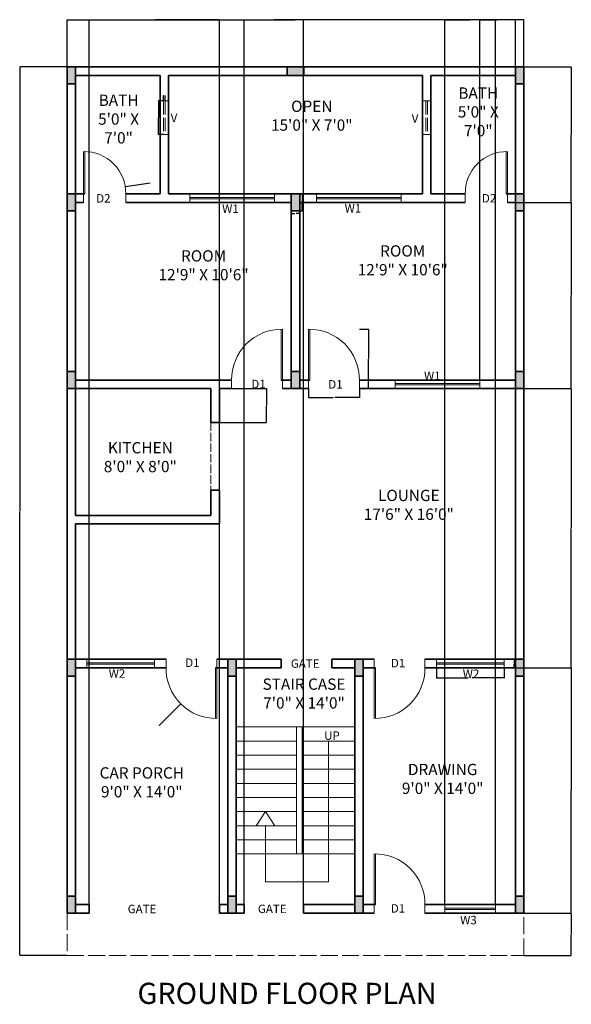
# Model space of a CAD drawing. Units: inches. Extents: x -1239 to -402, y 1021 to 1720.
# Tile 1 of 2: x -1239 to -847, y 1021 to 1720. Entities that reach past the tile are written whole.
import ezdxf

# ---------------------------------------------------------------- set-up
doc = ezdxf.new("R2010")
doc.units = ezdxf.units.IN
doc.linetypes.add('ACAD_ISO02W100', pattern=[15, 12, -3])
for name, color, linetype, lineweight in [('A-ANNO-DIMS', 2, 'Continuous', 18), ('A-ANNO-SYMB', 7, 'Continuous', 18), ('A-ANNO-TEXT', 7, 'Continuous', 18), ('A-ANNO-TITL', 7, 'Continuous', 35), ('A-AREA-IDEN', 7, 'Continuous', 18), ('A-COLS', 7, 'Continuous', 35), ('A-DOOR', 3, 'Continuous', 18), ('A-FLOR-OVHD', 8, 'ACAD_ISO02W100', 18), ('A-FLOR-STRS', 7, 'Continuous', 18), ('A-GLAZ', 4, 'Continuous', 18), ('A-GLAZ-HIDN', 4, 'ACAD_ISO02W100', 13), ('A-WALL', 7, 'Continuous', 35), ('A-WALL-OVHD', 8, 'ACAD_ISO02W100', 18)]:
    doc.layers.add(name, color=color, linetype=linetype, lineweight=lineweight)
doc.styles.get("Standard").update_dxf_attribs({"font": 'arial.ttf'})
doc.dimstyles.get("Standard").update_dxf_attribs({"dimtxt": 0.18, "dimasz": 0.18, "dimexe": 0.18, "dimexo": 0.0625, "dimgap": 0.09, "dimtad": 0, "dimtih": 1, "dimtoh": 1, "dimdec": 4, "dimzin": 0, "dimdsep": 46, "dimtxsty": 'Standard', "dimcen": 0.09, "dimadec": 0, "dimazin": 0, "dimtfac": 1, "dimtdec": 4, "dimtofl": 0, "dimtmove": 0, "dimatfit": 3, "dimfxl": 1, "dimtolj": 1, "dimtzin": 0, "dimarcsym": 0})

# ---------------------------------------------------------------- blocks, each defined once
blk = doc.blocks.new('DOOR-D1-36IN')
for p, q in [((0, 0), (0, 36)), ((1, 0), (1, 36)), ((0, 0), (0, -6)), ((36, 0), (36, -6))]:
    blk.add_line(p, q)
blk.add_arc((0.5, 0.5), 35.5, 359.19307, 90.80693)
blk = doc.blocks.new('DOOR-D2-30IN')
for p, q in [((0, 0), (0, 30)), ((1, 0), (1, 30)), ((0, 0), (0, -6)), ((30, 0), (30, -6))]:
    blk.add_line(p, q)
blk.add_arc((0.5, 0.5), 29.5, 359.02898, 90.97102)
blk = doc.blocks.new('WINDOW-W1-60IN')
for p, q in [((0, 0), (0, -6)), ((60, 0), (60, -6)), ((0, -2.5), (60, -2.5)), ((0, -3.5), (60, -3.5))]:
    blk.add_line(p, q)
blk = doc.blocks.new('WINDOW-W2-48IN')
for p, q in [((0, 0), (0, 6)), ((0, 3.5), (48, 3.5)), ((0, 2.5), (48, 2.5)), ((48, 0), (48, 6))]:
    blk.add_line(p, q)
blk = doc.blocks.new('COLUMN-6X12IN')
h = blk.add_hatch(color=256)
h.dxf.hatch_style = 1
h.paths.add_polyline_path([(6, 12), (0, 12), (0, 0), (6, 0)])
for p, q in [((0, 12), (6, 12)), ((0, 0), (0, 12)), ((6, 12), (6, 0)), ((6, 0), (0, 0))]:
    blk.add_line(p, q)
blk = doc.blocks.new('VENT-SASH-24IN')
at = {"ltscale": 0.8}
for p, q in [((0, 0), (0, -24)), ((1, 0), (1, -24))]:
    blk.add_line(p, q, dxfattribs=at)
blk = doc.blocks.new('*D7')
at = {"layer": 'A-ANNO-DIMS', "color": 0, "lineweight": -2, "transparency": 16777216}
for p, q in [((-1039.91, 1596.03), (-1038, 1596.03)), ((-1038.18, 1595.85), (-1038.18, 1590.21)), ((-1038.18, 1584.21), (-1038.18, 1589.84)), ((-1039.91, 1584.03), (-1038, 1584.03))]:
    blk.add_line(p, q, dxfattribs=at)
at = {"layer": 'A-ANNO-DIMS', "color": 0, "transparency": 16777216}
for points in [[(-1038.21, 1595.85), (-1038.15, 1595.85), (-1038.18, 1596.03)], [(-1038.21, 1584.21), (-1038.15, 1584.21), (-1038.18, 1584.03)]]:
    blk.add_solid(points, dxfattribs=at)
at = {"layer": 'Defpoints', "color": 0, "transparency": 16777216}
for p in [(-1039.98, 1596.03), (-1038.18, 1596.03), (-1039.98, 1584.03)]:
    blk.add_point(p, dxfattribs=at)
at = {"layer": 'A-ANNO-DIMS', "color": 0, "transparency": 16777216, "insert": (-1038.18, 1590.03), "char_height": 0.18, "attachment_point": 5}
blk.add_mtext('\\A1;COLUMN 12 TYP.', dxfattribs=at)
blk = doc.blocks.new('*D8')
at = {"layer": 'A-ANNO-DIMS', "color": 0, "lineweight": -2, "transparency": 16777216}
for p, q in [((-1045.98, 1583.97), (-1045.98, 1582.05)), ((-1045.8, 1582.23), (-1043.44, 1582.23)), ((-1040.16, 1582.23), (-1042.52, 1582.23)), ((-1039.98, 1583.97), (-1039.98, 1582.05))]:
    blk.add_line(p, q, dxfattribs=at)
at = {"layer": 'A-ANNO-DIMS', "color": 0, "transparency": 16777216}
for points in [[(-1045.8, 1582.26), (-1045.8, 1582.2), (-1045.98, 1582.23)], [(-1040.16, 1582.26), (-1040.16, 1582.2), (-1039.98, 1582.23)]]:
    blk.add_solid(points, dxfattribs=at)
at = {"layer": 'Defpoints', "color": 0, "transparency": 16777216}
for p in [(-1045.98, 1584.03), (-1039.98, 1584.03), (-1039.98, 1582.23)]:
    blk.add_point(p, dxfattribs=at)
at = {"layer": 'A-ANNO-DIMS', "color": 0, "transparency": 16777216, "insert": (-1042.98, 1582.23), "char_height": 0.18, "attachment_point": 5}
blk.add_mtext('\\A1;6 TYP.', dxfattribs=at)
blk = doc.blocks.new('*D9')
at = {"layer": 'A-ANNO-DIMS', "color": 0, "lineweight": -2, "transparency": 16777216}
for p, q in [((-997.51, 1500.16), (-991.08, 1500.16)), ((-991.26, 1499.98), (-991.26, 1479.28)), ((-991.26, 1458.21), (-991.26, 1478.91)), ((-997.51, 1458.03), (-991.08, 1458.03))]:
    blk.add_line(p, q, dxfattribs=at)
at = {"layer": 'A-ANNO-DIMS', "color": 0, "transparency": 16777216}
for points in [[(-991.29, 1499.98), (-991.23, 1499.98), (-991.26, 1500.16)], [(-991.29, 1458.21), (-991.23, 1458.21), (-991.26, 1458.03)]]:
    blk.add_solid(points, dxfattribs=at)
at = {"layer": 'Defpoints', "color": 0, "transparency": 16777216}
for p in [(-997.58, 1500.16), (-991.26, 1500.16), (-997.58, 1458.03)]:
    blk.add_point(p, dxfattribs=at)
at = {"layer": 'A-ANNO-DIMS', "color": 0, "transparency": 16777216, "insert": (-991.26, 1479.1), "char_height": 0.18, "attachment_point": 5}
blk.add_mtext('\\A1;DOOR D1 42 TYP.', dxfattribs=at)
blk = doc.blocks.new('*D10')
at = {"layer": 'A-ANNO-DIMS', "color": 0, "lineweight": -2, "transparency": 16777216}
for p, q in [((-1033.71, 1457.97), (-1033.71, 1451.53)), ((-997.58, 1457.97), (-997.58, 1451.53)), ((-1033.53, 1451.71), (-1016.17, 1451.71)), ((-997.76, 1451.71), (-1015.12, 1451.71))]:
    blk.add_line(p, q, dxfattribs=at)
at = {"layer": 'A-ANNO-DIMS', "color": 0, "transparency": 16777216}
for points in [[(-1033.53, 1451.74), (-1033.53, 1451.68), (-1033.71, 1451.71)], [(-997.76, 1451.74), (-997.76, 1451.68), (-997.58, 1451.71)]]:
    blk.add_solid(points, dxfattribs=at)
at = {"layer": 'Defpoints', "color": 0, "transparency": 16777216}
for p in [(-1033.71, 1458.03), (-997.58, 1458.03), (-997.58, 1451.71)]:
    blk.add_point(p, dxfattribs=at)
at = {"layer": 'A-ANNO-DIMS', "color": 0, "transparency": 16777216, "insert": (-1015.64, 1451.71), "char_height": 0.18, "attachment_point": 5}
blk.add_mtext('\\A1;36 TYP.', dxfattribs=at)
blk = doc.blocks.new('*D15')
at = {"layer": 'A-ANNO-DIMS', "color": 0, "lineweight": -2, "transparency": 16777216}
for p, q in [((-943.1, 1259.97), (-943.1, 1252.65)), ((-895.1, 1259.97), (-895.1, 1252.65)), ((-942.92, 1252.83), (-920.44, 1252.83)), ((-895.28, 1252.83), (-917.76, 1252.83))]:
    blk.add_line(p, q, dxfattribs=at)
at = {"layer": 'A-ANNO-DIMS', "color": 0, "transparency": 16777216}
for points in [[(-942.92, 1252.86), (-942.92, 1252.8), (-943.1, 1252.83)], [(-895.28, 1252.86), (-895.28, 1252.8), (-895.1, 1252.83)]]:
    blk.add_solid(points, dxfattribs=at)
at = {"layer": 'Defpoints', "color": 0, "transparency": 16777216}
for p in [(-943.1, 1260.03), (-895.1, 1260.03), (-895.1, 1252.83)]:
    blk.add_point(p, dxfattribs=at)
at = {"layer": 'A-ANNO-DIMS', "color": 0, "transparency": 16777216, "insert": (-919.1, 1252.83), "char_height": 0.18, "attachment_point": 5}
blk.add_mtext('\\A1;WINDOW W2 48 TYP.', dxfattribs=at)
blk = doc.blocks.new('*D16')
at = {"layer": 'A-ANNO-DIMS', "color": 0, "lineweight": -2, "transparency": 16777216}
for p, q in [((-895.03, 1266.03), (-887.72, 1266.03)), ((-887.9, 1265.85), (-887.9, 1263.21)), ((-895.03, 1260.03), (-887.72, 1260.03)), ((-887.9, 1260.21), (-887.9, 1262.85))]:
    blk.add_line(p, q, dxfattribs=at)
at = {"layer": 'A-ANNO-DIMS', "color": 0, "transparency": 16777216}
for points in [[(-887.93, 1265.85), (-887.87, 1265.85), (-887.9, 1266.03)], [(-887.93, 1260.21), (-887.87, 1260.21), (-887.9, 1260.03)]]:
    blk.add_solid(points, dxfattribs=at)
at = {"layer": 'Defpoints', "color": 0, "transparency": 16777216}
for p in [(-895.1, 1266.03), (-887.9, 1266.03), (-895.1, 1260.03)]:
    blk.add_point(p, dxfattribs=at)
at = {"layer": 'A-ANNO-DIMS', "color": 0, "transparency": 16777216, "insert": (-887.9, 1263.03), "char_height": 0.18, "attachment_point": 5}
blk.add_mtext('\\A1;6 TYP.', dxfattribs=at)
blk = doc.blocks.new('*D17')
at = {"layer": 'A-ANNO-DIMS', "color": 0, "lineweight": -2, "transparency": 16777216}
for p, q in [((-1136.54, 1662.03), (-1140.26, 1662.03)), ((-1140.08, 1661.85), (-1140.08, 1650.21)), ((-1140.08, 1638.21), (-1140.08, 1649.85)), ((-1136.54, 1638.03), (-1140.26, 1638.03))]:
    blk.add_line(p, q, dxfattribs=at)
at = {"layer": 'A-ANNO-DIMS', "color": 0, "transparency": 16777216}
for points in [[(-1140.11, 1661.85), (-1140.05, 1661.85), (-1140.08, 1662.03)], [(-1140.11, 1638.21), (-1140.05, 1638.21), (-1140.08, 1638.03)]]:
    blk.add_solid(points, dxfattribs=at)
at = {"layer": 'Defpoints', "color": 0, "transparency": 16777216}
for p in [(-1140.08, 1662.03), (-1136.48, 1662.03), (-1136.48, 1638.03)]:
    blk.add_point(p, dxfattribs=at)
at = {"layer": 'A-ANNO-DIMS', "color": 0, "transparency": 16777216, "insert": (-1140.08, 1650.03), "char_height": 0.18, "attachment_point": 5}
blk.add_mtext('\\A1;VENT 24 TYP.', dxfattribs=at)
blk = doc.blocks.new('*D18')
at = {"layer": 'A-ANNO-DIMS', "color": 0, "lineweight": -2, "transparency": 16777216}
for p, q in [((-1136.66, 1665.63), (-1136.84, 1665.63)), ((-1136.48, 1662.09), (-1136.48, 1665.81)), ((-1135.48, 1662.09), (-1135.48, 1665.81)), ((-1135.3, 1665.63), (-1135.12, 1665.63))]:
    blk.add_line(p, q, dxfattribs=at)
at = {"layer": 'A-ANNO-DIMS', "color": 0, "transparency": 16777216}
for points in [[(-1136.66, 1665.66), (-1136.66, 1665.6), (-1136.48, 1665.63)], [(-1135.3, 1665.66), (-1135.3, 1665.6), (-1135.48, 1665.63)]]:
    blk.add_solid(points, dxfattribs=at)
at = {"layer": 'Defpoints', "color": 0, "transparency": 16777216}
for p in [(-1136.48, 1662.03), (-1135.48, 1665.63), (-1135.48, 1662.03)]:
    blk.add_point(p, dxfattribs=at)
at = {"layer": 'A-ANNO-DIMS', "color": 0, "transparency": 16777216, "insert": (-1135.98, 1665.63), "char_height": 0.18, "attachment_point": 5}
blk.add_mtext('\\A1;1 TYP.', dxfattribs=at)
blk = doc.blocks.new('*D19')
at = {"layer": 'A-ANNO-DIMS', "color": 0, "lineweight": -2, "transparency": 16777216}
for p, q in [((-1204.98, 1686.09), (-1204.98, 1719.56)), ((-1204.8, 1719.38), (-1043.27, 1719.38)), ((-881.16, 1719.38), (-1042.69, 1719.38)), ((-880.98, 1686.09), (-880.98, 1719.56))]:
    blk.add_line(p, q, dxfattribs=at)
at = {"layer": 'A-ANNO-DIMS', "color": 0, "transparency": 16777216}
for points in [[(-1204.8, 1719.41), (-1204.8, 1719.35), (-1204.98, 1719.38)], [(-881.16, 1719.41), (-881.16, 1719.35), (-880.98, 1719.38)]]:
    blk.add_solid(points, dxfattribs=at)
at = {"layer": 'Defpoints', "color": 0, "transparency": 16777216}
for p in [(-880.98, 1719.38), (-1204.98, 1686.03), (-880.98, 1686.03)]:
    blk.add_point(p, dxfattribs=at)
at = {"layer": 'A-ANNO-DIMS', "color": 0, "transparency": 16777216, "insert": (-1042.98, 1719.38), "char_height": 0.18, "attachment_point": 5}
blk.add_mtext('\\A1;324', dxfattribs=at)
blk = doc.blocks.new('*D20')
at = {"layer": 'A-ANNO-DIMS', "color": 0, "lineweight": -2, "transparency": 16777216}
for p, q in [((-1205.04, 1686.03), (-1238.51, 1686.03)), ((-1238.33, 1685.85), (-1238.33, 1371.21)), ((-1238.33, 1056.21), (-1238.33, 1370.85)), ((-1205.04, 1056.03), (-1238.51, 1056.03))]:
    blk.add_line(p, q, dxfattribs=at)
at = {"layer": 'A-ANNO-DIMS', "color": 0, "transparency": 16777216}
for points in [[(-1238.36, 1685.85), (-1238.3, 1685.85), (-1238.33, 1686.03)], [(-1238.36, 1056.21), (-1238.3, 1056.21), (-1238.33, 1056.03)]]:
    blk.add_solid(points, dxfattribs=at)
at = {"layer": 'Defpoints', "color": 0, "transparency": 16777216}
for p in [(-1238.33, 1686.03), (-1204.98, 1686.03), (-1204.98, 1056.03)]:
    blk.add_point(p, dxfattribs=at)
at = {"layer": 'A-ANNO-DIMS', "color": 0, "transparency": 16777216, "insert": (-1238.33, 1371.03), "char_height": 0.18, "attachment_point": 5}
blk.add_mtext('\\A1;630', dxfattribs=at)
blk = doc.blocks.new('*D23')
at = {"layer": 'A-ANNO-DIMS', "color": 0, "lineweight": -2, "transparency": 16777216}
for p, q in [((-880.91, 1086.03), (-847.45, 1086.03)), ((-847.63, 1085.85), (-847.63, 1071.21)), ((-847.63, 1056.21), (-847.63, 1070.85)), ((-880.91, 1056.03), (-847.45, 1056.03))]:
    blk.add_line(p, q, dxfattribs=at)
at = {"layer": 'A-ANNO-DIMS', "color": 0, "transparency": 16777216}
for points in [[(-847.66, 1085.85), (-847.6, 1085.85), (-847.63, 1086.03)], [(-847.66, 1056.21), (-847.6, 1056.21), (-847.63, 1056.03)]]:
    blk.add_solid(points, dxfattribs=at)
at = {"layer": 'Defpoints', "color": 0, "transparency": 16777216}
for p in [(-880.98, 1086.03), (-847.63, 1086.03), (-880.98, 1056.03)]:
    blk.add_point(p, dxfattribs=at)
at = {"layer": 'A-ANNO-DIMS', "color": 0, "transparency": 16777216, "insert": (-847.63, 1071.03), "char_height": 0.18, "attachment_point": 5}
blk.add_mtext('\\A1;30', dxfattribs=at)
blk = doc.blocks.new('*D24')
at = {"layer": 'A-ANNO-DIMS', "color": 0, "lineweight": -2, "transparency": 16777216}
for p, q in [((-886.91, 1260.03), (-847.45, 1260.03)), ((-847.63, 1259.85), (-847.63, 1173.21)), ((-847.63, 1086.21), (-847.63, 1172.85)), ((-880.91, 1086.03), (-847.45, 1086.03))]:
    blk.add_line(p, q, dxfattribs=at)
at = {"layer": 'A-ANNO-DIMS', "color": 0, "transparency": 16777216}
for points in [[(-847.66, 1259.85), (-847.6, 1259.85), (-847.63, 1260.03)], [(-847.66, 1086.21), (-847.6, 1086.21), (-847.63, 1086.03)]]:
    blk.add_solid(points, dxfattribs=at)
at = {"layer": 'Defpoints', "color": 0, "transparency": 16777216}
for p in [(-886.98, 1260.03), (-847.63, 1260.03), (-880.98, 1086.03)]:
    blk.add_point(p, dxfattribs=at)
at = {"layer": 'A-ANNO-DIMS', "color": 0, "transparency": 16777216, "insert": (-847.63, 1173.03), "char_height": 0.18, "attachment_point": 5}
blk.add_mtext('\\A1;174', dxfattribs=at)
blk = doc.blocks.new('*D25')
at = {"layer": 'A-ANNO-DIMS', "color": 0, "lineweight": -2, "transparency": 16777216}
for p, q in [((-880.91, 1458.03), (-847.45, 1458.03)), ((-847.63, 1457.85), (-847.63, 1359.21)), ((-847.63, 1260.21), (-847.63, 1358.85)), ((-886.91, 1260.03), (-847.45, 1260.03))]:
    blk.add_line(p, q, dxfattribs=at)
at = {"layer": 'A-ANNO-DIMS', "color": 0, "transparency": 16777216}
for points in [[(-847.66, 1457.85), (-847.6, 1457.85), (-847.63, 1458.03)], [(-847.66, 1260.21), (-847.6, 1260.21), (-847.63, 1260.03)]]:
    blk.add_solid(points, dxfattribs=at)
at = {"layer": 'Defpoints', "color": 0, "transparency": 16777216}
for p in [(-880.98, 1458.03), (-847.63, 1458.03), (-886.98, 1260.03)]:
    blk.add_point(p, dxfattribs=at)
at = {"layer": 'A-ANNO-DIMS', "color": 0, "transparency": 16777216, "insert": (-847.63, 1359.03), "char_height": 0.18, "attachment_point": 5}
blk.add_mtext('\\A1;198', dxfattribs=at)
blk = doc.blocks.new('*D26')
at = {"layer": 'A-ANNO-DIMS', "color": 0, "lineweight": -2, "transparency": 16777216}
for p, q in [((-886.91, 1590.03), (-847.45, 1590.03)), ((-847.63, 1589.85), (-847.63, 1524.21)), ((-847.63, 1458.21), (-847.63, 1523.85)), ((-880.91, 1458.03), (-847.45, 1458.03))]:
    blk.add_line(p, q, dxfattribs=at)
at = {"layer": 'A-ANNO-DIMS', "color": 0, "transparency": 16777216}
for points in [[(-847.66, 1589.85), (-847.6, 1589.85), (-847.63, 1590.03)], [(-847.66, 1458.21), (-847.6, 1458.21), (-847.63, 1458.03)]]:
    blk.add_solid(points, dxfattribs=at)
at = {"layer": 'Defpoints', "color": 0, "transparency": 16777216}
for p in [(-886.98, 1590.03), (-847.63, 1590.03), (-880.98, 1458.03)]:
    blk.add_point(p, dxfattribs=at)
at = {"layer": 'A-ANNO-DIMS', "color": 0, "transparency": 16777216, "insert": (-847.63, 1524.03), "char_height": 0.18, "attachment_point": 5}
blk.add_mtext('\\A1;132', dxfattribs=at)
blk = doc.blocks.new('*D27')
at = {"layer": 'A-ANNO-DIMS', "color": 0, "lineweight": -2, "transparency": 16777216}
for p, q in [((-880.91, 1686.03), (-847.45, 1686.03)), ((-847.63, 1685.85), (-847.63, 1638.21)), ((-847.63, 1590.21), (-847.63, 1637.85)), ((-886.91, 1590.03), (-847.45, 1590.03))]:
    blk.add_line(p, q, dxfattribs=at)
at = {"layer": 'A-ANNO-DIMS', "color": 0, "transparency": 16777216}
for points in [[(-847.66, 1685.85), (-847.6, 1685.85), (-847.63, 1686.03)], [(-847.66, 1590.21), (-847.6, 1590.21), (-847.63, 1590.03)]]:
    blk.add_solid(points, dxfattribs=at)
at = {"layer": 'Defpoints', "color": 0, "transparency": 16777216}
for p in [(-880.98, 1686.03), (-847.63, 1686.03), (-886.98, 1590.03)]:
    blk.add_point(p, dxfattribs=at)
at = {"layer": 'A-ANNO-DIMS', "color": 0, "transparency": 16777216, "insert": (-847.63, 1638.03), "char_height": 0.18, "attachment_point": 5}
blk.add_mtext('\\A1;96', dxfattribs=at)
blk = doc.blocks.new('*D28')
at = {"layer": 'A-ANNO-DIMS', "color": 0, "lineweight": -2, "transparency": 16777216}
for p, q in [((-1189.23, 1092.09), (-1189.23, 1719.56)), ((-1189.05, 1719.38), (-1143.43, 1719.38)), ((-1097.02, 1719.38), (-1142.64, 1719.38)), ((-1096.84, 1092.09), (-1096.84, 1719.56))]:
    blk.add_line(p, q, dxfattribs=at)
at = {"layer": 'A-ANNO-DIMS', "color": 0, "transparency": 16777216}
for points in [[(-1189.05, 1719.41), (-1189.05, 1719.35), (-1189.23, 1719.38)], [(-1097.02, 1719.41), (-1097.02, 1719.35), (-1096.84, 1719.38)]]:
    blk.add_solid(points, dxfattribs=at)
at = {"layer": 'Defpoints', "color": 0, "transparency": 16777216}
for p in [(-1096.84, 1719.38), (-1189.23, 1092.03), (-1096.84, 1092.03)]:
    blk.add_point(p, dxfattribs=at)
at = {"layer": 'A-ANNO-DIMS', "color": 0, "transparency": 16777216, "insert": (-1143.03, 1719.38), "char_height": 0.18, "attachment_point": 5}
blk.add_mtext('\\A1;92.39', dxfattribs=at)
blk = doc.blocks.new('*D29')
at = {"layer": 'A-ANNO-DIMS', "color": 0, "lineweight": -2, "transparency": 16777216}
for p, q in [((-1079.36, 1092.09), (-1079.36, 1719.56)), ((-1079.18, 1719.38), (-1058.58, 1719.38)), ((-1037.54, 1719.38), (-1058.14, 1719.38)), ((-1037.36, 1092.09), (-1037.36, 1719.56))]:
    blk.add_line(p, q, dxfattribs=at)
at = {"layer": 'A-ANNO-DIMS', "color": 0, "transparency": 16777216}
for points in [[(-1079.18, 1719.41), (-1079.18, 1719.35), (-1079.36, 1719.38)], [(-1037.54, 1719.41), (-1037.54, 1719.35), (-1037.36, 1719.38)]]:
    blk.add_solid(points, dxfattribs=at)
at = {"layer": 'Defpoints', "color": 0, "transparency": 16777216}
for p in [(-1037.36, 1719.38), (-1079.36, 1092.03), (-1037.36, 1092.03)]:
    blk.add_point(p, dxfattribs=at)
at = {"layer": 'A-ANNO-DIMS', "color": 0, "transparency": 16777216, "insert": (-1058.36, 1719.38), "char_height": 0.18, "attachment_point": 5}
blk.add_mtext('\\A1;42', dxfattribs=at)
blk = doc.blocks.new('*D30')
at = {"layer": 'A-ANNO-DIMS', "color": 0, "lineweight": -2, "transparency": 16777216}
for p, q in [((-937.1, 1092.09), (-937.1, 1719.56)), ((-936.92, 1719.38), (-919.32, 1719.38)), ((-901.28, 1719.38), (-918.88, 1719.38)), ((-901.1, 1092.09), (-901.1, 1719.56))]:
    blk.add_line(p, q, dxfattribs=at)
at = {"layer": 'A-ANNO-DIMS', "color": 0, "transparency": 16777216}
for points in [[(-936.92, 1719.41), (-936.92, 1719.35), (-937.1, 1719.38)], [(-901.28, 1719.41), (-901.28, 1719.35), (-901.1, 1719.38)]]:
    blk.add_solid(points, dxfattribs=at)
at = {"layer": 'Defpoints', "color": 0, "transparency": 16777216}
for p in [(-901.1, 1719.38), (-937.1, 1092.03), (-901.1, 1092.03)]:
    blk.add_point(p, dxfattribs=at)
at = {"layer": 'A-ANNO-DIMS', "color": 0, "transparency": 16777216, "insert": (-919.1, 1719.38), "char_height": 0.18, "attachment_point": 5}
blk.add_mtext('\\A1;36', dxfattribs=at)
blk = doc.blocks.new('*D36')
at = {"layer": 'A-ANNO-DIMS', "color": 0, "lineweight": -2, "transparency": 16777216}
for p, q in [((-1096.91, 1458.03), (-1063.45, 1458.03)), ((-1063.63, 1457.85), (-1063.63, 1446.21)), ((-1063.63, 1434.21), (-1063.63, 1445.85)), ((-1096.91, 1434.03), (-1063.45, 1434.03))]:
    blk.add_line(p, q, dxfattribs=at)
at = {"layer": 'A-ANNO-DIMS', "color": 0, "transparency": 16777216}
for points in [[(-1063.66, 1457.85), (-1063.6, 1457.85), (-1063.63, 1458.03)], [(-1063.66, 1434.21), (-1063.6, 1434.21), (-1063.63, 1434.03)]]:
    blk.add_solid(points, dxfattribs=at)
at = {"layer": 'Defpoints', "color": 0, "transparency": 16777216}
for p in [(-1096.98, 1458.03), (-1096.98, 1434.03), (-1063.63, 1434.03)]:
    blk.add_point(p, dxfattribs=at)
at = {"layer": 'A-ANNO-DIMS', "color": 0, "transparency": 16777216, "insert": (-1063.63, 1446.03), "char_height": 0.18, "attachment_point": 5}
blk.add_mtext('\\A1;24', dxfattribs=at)
blk = doc.blocks.new('*D38')
at = {"layer": 'A-ANNO-DIMS', "color": 0, "lineweight": -2, "transparency": 16777216}
for p, q in [((-912.34, 1464.09), (-912.34, 1719.56)), ((-912.16, 1719.38), (-900.13, 1719.38)), ((-887.16, 1719.38), (-899.2, 1719.38)), ((-886.98, 1464.09), (-886.98, 1719.56))]:
    blk.add_line(p, q, dxfattribs=at)
at = {"layer": 'A-ANNO-DIMS', "color": 0, "transparency": 16777216}
for points in [[(-912.16, 1719.41), (-912.16, 1719.35), (-912.34, 1719.38)], [(-887.16, 1719.41), (-887.16, 1719.35), (-886.98, 1719.38)]]:
    blk.add_solid(points, dxfattribs=at)
at = {"layer": 'Defpoints', "color": 0, "transparency": 16777216}
for p in [(-886.98, 1719.38), (-912.34, 1464.03), (-886.98, 1464.03)]:
    blk.add_point(p, dxfattribs=at)
at = {"layer": 'A-ANNO-DIMS', "color": 0, "transparency": 16777216, "insert": (-899.66, 1719.38), "char_height": 0.18, "attachment_point": 5}
blk.add_mtext('\\A1;25.367', dxfattribs=at)
blk = doc.blocks.new('*D39')
at = {"layer": 'A-ANNO-DIMS', "color": 0, "lineweight": -2, "transparency": 16777216}
for p, q in [((-1099.33, 1259.53), (-1099.15, 1259.53)), ((-1099.24, 1259.44), (-1099.24, 1259.62)), ((-1139.41, 1219.36), (-1124.47, 1234.3)), ((-1139.59, 1219.36), (-1139.41, 1219.36))]:
    blk.add_line(p, q, dxfattribs=at)
at = {"layer": 'A-ANNO-DIMS', "color": 0, "transparency": 16777216}
blk.add_solid([(-1124.49, 1234.32), (-1124.45, 1234.27), (-1124.34, 1234.42)], dxfattribs=at)
at = {"layer": 'Defpoints', "color": 0, "transparency": 16777216}
for p in [(-1099.24, 1259.53), (-1124.34, 1234.42)]:
    blk.add_point(p, dxfattribs=at)
at = {"layer": 'A-ANNO-DIMS', "color": 0, "transparency": 16777216, "insert": (-1140.19, 1219.36), "char_height": 0.18, "attachment_point": 5}
blk.add_mtext('\\A1;5X R35.5', dxfattribs=at)
blk = doc.blocks.new('*D40')
at = {"layer": 'A-ANNO-DIMS', "color": 0, "lineweight": -2, "transparency": 16777216}
for p, q in [((-1146.14, 1603.53), (-1163.47, 1600.93)), ((-1192.91, 1596.53), (-1192.73, 1596.53)), ((-1192.82, 1596.44), (-1192.82, 1596.62))]:
    blk.add_line(p, q, dxfattribs=at)
at = {"layer": 'A-ANNO-DIMS', "color": 0, "transparency": 16777216}
blk.add_solid([(-1163.47, 1600.96), (-1163.46, 1600.9), (-1163.64, 1600.9)], dxfattribs=at)
at = {"layer": 'Defpoints', "color": 0, "transparency": 16777216}
for p in [(-1163.64, 1600.9), (-1192.82, 1596.53)]:
    blk.add_point(p, dxfattribs=at)
at = {"layer": 'A-ANNO-DIMS', "color": 0, "transparency": 16777216, "insert": (-1145.39, 1603.53), "char_height": 0.18, "attachment_point": 5}
blk.add_mtext('\\A1;2X R29.504', dxfattribs=at)

msp = doc.modelspace()

# ---------------------------------------------------------------- linework, layer by layer
at = {"layer": 'A-ANNO-SYMB'}
for p, q in [((-1019.5728, 1208.028), (-1019.5728, 1108.2999)), ((-1064.2192, 1158.028), (-1070.9011, 1148.028)), ((-1064.2192, 1158.028), (-1057.5374, 1148.028)), ((-1064.2192, 1108.2999), (-1064.2192, 1148.028)), ((-1019.5728, 1108.2999), (-1064.2192, 1108.2999))]:
    msp.add_line(p, q, dxfattribs=at)
at = {"layer": 'A-FLOR-OVHD'}
for p, q in [((-1204.9774, 1086.028), (-1204.9774, 1056.028)), ((-880.9774, 1056.028), (-880.9774, 1086.028)), ((-1204.9774, 1056.028), (-880.9774, 1056.028))]:
    msp.add_line(p, q, dxfattribs=at)
at = {"layer": 'A-FLOR-STRS'}
for p, q in [((-1084.9774, 1218.028), (-1042.1682, 1218.028)), ((-1042.1682, 1128.028), (-1042.1682, 1218.028)), ((-1042.1682, 1218.028), (-1000.9774, 1218.028)), ((-1038.1682, 1128.028), (-1038.1682, 1218.028)), ((-1084.9774, 1208.028), (-1042.1682, 1208.028)), ((-1038.1682, 1208.028), (-1000.9774, 1208.028)), ((-1084.9774, 1198.028), (-1042.1682, 1198.028)), ((-1038.1682, 1198.028), (-1000.9774, 1198.028)), ((-1084.9774, 1188.028), (-1042.1682, 1188.028)), ((-1038.1682, 1188.028), (-1000.9774, 1188.028)), ((-1084.9774, 1178.028), (-1042.1682, 1178.028)), ((-1038.1682, 1178.028), (-1000.9774, 1178.028)), ((-1084.9774, 1168.028), (-1042.1682, 1168.028)), ((-1038.1682, 1168.028), (-1000.9774, 1168.028)), ((-1084.9774, 1158.028), (-1042.1682, 1158.028)), ((-1038.1682, 1158.028), (-1000.9774, 1158.028)), ((-1084.9774, 1148.028), (-1042.1682, 1148.028)), ((-1038.1682, 1148.028), (-1000.9774, 1148.028)), ((-1084.9774, 1138.028), (-1042.1682, 1138.028)), ((-1038.1682, 1138.028), (-1000.9774, 1138.028)), ((-1084.9774, 1128.028), (-1042.1682, 1128.028)), ((-1042.1682, 1128.028), (-1000.9774, 1128.028))]:
    msp.add_line(p, q, dxfattribs=at)
at = {"layer": 'A-GLAZ'}
for p, q in [((-1138.9774, 1662.028), (-1132.9774, 1662.028)), ((-952.9774, 1662.028), (-946.9774, 1662.028)), ((-1138.9774, 1638.028), (-1132.9774, 1638.028)), ((-952.9774, 1638.028), (-946.9774, 1638.028)), ((-937.0971, 1092.028), (-937.0971, 1086.028)), ((-937.0971, 1089.528), (-901.0971, 1089.528)), ((-901.0971, 1092.028), (-901.0971, 1086.028)), ((-937.0971, 1088.528), (-901.0971, 1088.528))]:
    msp.add_line(p, q, dxfattribs=at)
at = {"layer": 'A-WALL'}
for p, q in [((-880.9774, 1686.028), (-1204.9774, 1686.028)), ((-1204.9774, 1686.028), (-1204.9774, 1086.028)), ((-880.9774, 1086.028), (-880.9774, 1686.028)), ((-1198.9774, 1680.028), (-1198.9774, 1596.028)), ((-1138.9774, 1680.028), (-1198.9774, 1680.028)), ((-1138.9774, 1680.028), (-1138.9774, 1596.028)), ((-1132.9774, 1680.028), (-1132.9774, 1596.028)), ((-952.9774, 1680.028), (-1132.9774, 1680.028)), ((-952.9774, 1596.028), (-952.9774, 1680.028)), ((-886.9774, 1680.028), (-946.9774, 1680.028)), ((-946.9774, 1596.028), (-946.9774, 1680.028)), ((-886.9774, 1596.028), (-886.9774, 1680.028)), ((-1198.9774, 1596.028), (-1192.3228, 1596.028)), ((-1163.3228, 1596.028), (-1138.9774, 1596.028)), ((-1132.9774, 1596.028), (-952.9774, 1596.028)), ((-946.9774, 1596.028), (-922.632, 1596.028)), ((-893.632, 1596.028), (-886.9774, 1596.028)), ((-1198.9774, 1590.028), (-1193.3228, 1590.028)), ((-1198.9774, 1590.028), (-1198.9774, 1464.028)), ((-1163.3228, 1590.028), (-1045.9774, 1590.028)), ((-1045.9774, 1590.028), (-1045.9774, 1464.028)), ((-1039.9774, 1464.028), (-1039.9774, 1590.028)), ((-1039.9774, 1590.028), (-922.632, 1590.028)), ((-892.632, 1590.028), (-886.9774, 1590.028)), ((-886.9774, 1464.028), (-886.9774, 1590.028)), ((-1198.9774, 1464.028), (-1088.2434, 1464.028)), ((-1053.2434, 1464.028), (-1045.9774, 1464.028)), ((-1039.9774, 1464.028), (-1032.7113, 1464.028)), ((-997.7113, 1464.028), (-886.9774, 1464.028)), ((-1198.9774, 1458.028), (-1102.9774, 1458.028)), ((-1198.9774, 1458.028), (-1198.9774, 1368.028)), ((-1102.9774, 1458.028), (-1102.9774, 1434.028)), ((-1096.9774, 1458.028), (-1096.9774, 1434.028)), ((-1096.9774, 1458.028), (-1088.2434, 1458.028)), ((-1052.2434, 1458.028), (-1033.7113, 1458.028)), ((-997.7113, 1458.028), (-886.9774, 1458.028)), ((-886.9774, 1266.028), (-886.9774, 1458.028)), ((-1096.9774, 1434.028), (-1102.9774, 1434.028)), ((-1096.9774, 1386.028), (-1102.9774, 1386.028)), ((-1102.9774, 1386.028), (-1102.9774, 1368.028)), ((-1096.9774, 1386.028), (-1096.9774, 1362.028)), ((-1198.9774, 1368.028), (-1102.9774, 1368.028)), ((-1198.9774, 1362.028), (-1096.9774, 1362.028)), ((-1198.9774, 1362.028), (-1198.9774, 1266.028)), ((-1198.9774, 1266.028), (-1134.7379, 1266.028)), ((-1098.7379, 1266.028), (-1053.1125, 1266.028)), ((-1053.1125, 1266.028), (-1053.1125, 1260.028)), ((-1017.1125, 1266.028), (-1017.1125, 1260.028)), ((-1017.1125, 1266.028), (-987.2168, 1266.028)), ((-951.2168, 1266.028), (-886.9774, 1266.028)), ((-1198.9774, 1260.028), (-1134.7379, 1260.028)), ((-1198.9774, 1260.028), (-1198.9774, 1092.028)), ((-1099.7379, 1260.028), (-1090.9774, 1260.028)), ((-1090.9774, 1260.028), (-1090.9774, 1092.028)), ((-1084.9774, 1260.028), (-1084.9774, 1092.028)), ((-1084.9774, 1260.028), (-1053.1125, 1260.028)), ((-1017.1125, 1260.028), (-1000.9774, 1260.028)), ((-1000.9774, 1092.028), (-1000.9774, 1260.028)), ((-994.9774, 1092.028), (-994.9774, 1260.028)), ((-994.9774, 1260.028), (-986.2168, 1260.028)), ((-951.2168, 1260.028), (-886.9774, 1260.028)), ((-886.9774, 1092.028), (-886.9774, 1260.028)), ((-1198.9774, 1092.028), (-1189.225, 1092.028)), ((-1189.225, 1092.028), (-1189.225, 1086.028)), ((-1096.8379, 1092.028), (-1096.8379, 1086.028)), ((-1096.8379, 1092.028), (-1090.9774, 1092.028)), ((-1084.9774, 1092.028), (-1079.359, 1092.028)), ((-1079.359, 1092.028), (-1079.359, 1086.028)), ((-1037.359, 1092.028), (-1037.359, 1086.028)), ((-1037.359, 1092.028), (-1000.9774, 1092.028)), ((-994.9774, 1092.028), (-986.2168, 1092.028)), ((-951.2168, 1092.028), (-886.9774, 1092.028)), ((-1204.9774, 1086.028), (-1189.225, 1086.028)), ((-1096.8379, 1086.028), (-1079.359, 1086.028)), ((-1037.359, 1086.028), (-987.2168, 1086.028)), ((-951.2168, 1086.028), (-880.9774, 1086.028))]:
    msp.add_line(p, q, dxfattribs=at)
at = {"layer": 'A-WALL-OVHD', "ltscale": 0.5}
for p, q in [((-1102.9774, 1434.028), (-1102.9774, 1386.028)), ((-1096.9774, 1434.028), (-1096.9774, 1386.028))]:
    msp.add_line(p, q, dxfattribs=at)

# ---------------------------------------------------------------- block references
at = {"layer": 'A-COLS'}
for p in [(-1204.9774, 1674.028), (-886.9774, 1674.028), (-1204.9774, 1584.028), (-1045.9774, 1584.028), (-886.9774, 1584.028), (-1204.9774, 1458.028), (-1045.9774, 1458.028), (-886.9774, 1458.028), (-1204.9774, 1254.028), (-1090.9774, 1254.028), (-1000.9774, 1254.028), (-886.9774, 1254.028), (-1204.9774, 1086.028), (-1090.9774, 1086.028), (-1000.9774, 1086.028), (-886.9774, 1086.028)]:
    msp.add_blockref('COLUMN-6X12IN', p, dxfattribs=at)
at = {"layer": 'A-COLS', "rotation": 89.9999999999984}
msp.add_blockref('COLUMN-6X12IN', (-1036.9774, 1680.028), dxfattribs=at)
at = {"layer": 'A-DOOR'}
for name, p in [('DOOR-D2-30IN', (-1193.3228, 1596.028)), ('DOOR-D1-36IN', (-1033.7113, 1464.028)), ('DOOR-D1-36IN', (-987.2168, 1092.028))]:
    msp.add_blockref(name, p, dxfattribs=at)
at = {"layer": 'A-DOOR', "extrusion": (0, 0, -1), "zscale": -1}
for name, p in [('DOOR-D2-30IN', (892.632, 1596.028)), ('DOOR-D1-36IN', (1052.2434, 1464.028))]:
    msp.add_blockref(name, p, dxfattribs=at)
at = {"layer": 'A-DOOR', "rotation": 180}
msp.add_blockref('DOOR-D1-36IN', (-1098.7379, 1260.028), dxfattribs=at)
at = {"layer": 'A-DOOR', "extrusion": (0, 0, -1), "zscale": -1, "rotation": 180}
msp.add_blockref('DOOR-D1-36IN', (987.2168, 1260.028), dxfattribs=at)
at = {"layer": 'A-GLAZ'}
for name, p in [('WINDOW-W1-60IN', (-1117.9752, 1596.028)), ('WINDOW-W2-48IN', (-1190.8576, 1260.028)), ('WINDOW-W2-48IN', (-943.0971, 1260.028))]:
    msp.add_blockref(name, p, dxfattribs=at)
at = {"layer": 'A-GLAZ', "rotation": 180}
for p in [(-967.9796, 1590.028), (-912.3443, 1458.028)]:
    msp.add_blockref('WINDOW-W1-60IN', p, dxfattribs=at)
at = {"layer": 'A-GLAZ-HIDN'}
for p in [(-1136.4774, 1662.028), (-950.4774, 1662.028)]:
    msp.add_blockref('VENT-SASH-24IN', p, dxfattribs=at)

# ---------------------------------------------------------------- texts
at = {"layer": 'A-ANNO-TEXT', "char_height": 6, "attachment_point": 1}
for s, width, insert in [('V', 21.819943, (-1131.5058, 1652.8943)), ('V', 21.819943, (-960.5924, 1652.5221)), ('D2', 21.819943, (-1184.3059, 1595.9048)), ('D2', 21.819943, (-910.8129, 1595.933)), ('W1', 21.819943, (-1094.9662, 1588.5129)), ('W1', 21.819943, (-1008.1035, 1588.7928)), ('W1', 21.819943, (-951.8414, 1470.0526)), ('D1', 21.819943, (-1074.2886, 1464.1788)), ('D1', 21.819943, (-1019.7447, 1464.0085)), ('D1', 21.819943, (-1121.1603, 1266.5784)), ('GATE', 57.104456, (-1046.2997, 1265.9537)), ('D1', 21.819943, (-975.3243, 1266.2834)), ('W2', 21.819943, (-1175.4045, 1258.8998)), ('W2', 21.819943, (-924.3943, 1258.7733)), ('UP', 21.819943, (-1022.6689, 1214.8762)), ('GATE', 57.104456, (-1161.9604, 1091.9481)), ('GATE', 57.104456, (-1069.6325, 1092.0227)), ('D1', 21.819943, (-975.3643, 1092.3524)), ('W3', 21.819943, (-926.2159, 1084.0836))]:
    msp.add_mtext_dynamic_manual_height_columns(s, width=width, gutter_width=12.5, heights=[0], dxfattribs=dict(at, insert=insert))
at = {"layer": 'A-ANNO-TITL', "insert": (-1193.1714, 1036.6182), "char_height": 15, "attachment_point": 1}
msp.add_mtext_dynamic_manual_height_columns('\\pxqc;{\\fArial|b1|i0|c0|p34;GROUND FLOOR PLAN}', width=288.409032, gutter_width=12.5, heights=[0], dxfattribs=at)
at = {"layer": 'A-AREA-IDEN', "char_height": 8, "attachment_point": 1}
for s, width, insert in [('\\pxqc;BATH\\P5\'0" X 7\'0"', 50.533842, (-938.6511, 1671.5305)), ('\\pxqc;BATH\\P5\'0" X 7\'0"', 50.533842, (-1193.681, 1666.432)), ('\\pxqc;OPEN\\P15\'0" X 7\'0"', 61.660387, (-1062.2681, 1662.1456)), ('\\pxqc;ROOM\\P12\'9" X 10\'6"', 86.734176, (-1010.314, 1559.5899)), ('\\pxqc;ROOM\\P12\'9" X 10\'6"', 86.734176, (-1151.5221, 1556.0826)), ('\\pxqc;KITCHEN\\P8\'0" X 8\'0"', 86.734176, (-1196.3755, 1420.0287)), ('\\pxqc;LOUNGE\\P17\'6" X 16\'0"', 86.734176, (-1005.9912, 1386.2223)), ('\\pxqc;STAIR CASE\\P7\'0" X 14\'0"', 86.734176, (-1080.3129, 1252.3765)), ('\\pxqc;CAR PORCH\\P9\'0" X 14\'0"', 86.734176, (-1195.3322, 1189.4315)), ('\\pxqc;DRAWING\\P9\'0" X 14\'0"', 86.734176, (-981.9982, 1191.8652))]:
    msp.add_mtext_dynamic_manual_height_columns(s, width=width, gutter_width=12.5, heights=[0], dxfattribs=dict(at, insert=insert))

# ---------------------------------------------------------------- dimensions: what is measured, and where the dimension line sits
at = {"layer": 'A-ANNO-DIMS'}
for base, p1, p2, override, picture, middle in [((-880.9774, 1719.378), (-1204.9774, 1686.028), (-880.9774, 1686.028), {"dimdec": 0, "dimlfac": 1, "dimrnd": 0, "dimzin": 0, "dimdsep": 46, "dimlunit": 2}, '*D19', (-1042.9774, 1719.378)), ((-1096.8379, 1719.378), (-1189.225, 1092.028), (-1096.8379, 1092.028), {"dimdec": 2, "dimlfac": 1, "dimrnd": 0, "dimzin": 0, "dimdsep": 46, "dimlunit": 2}, '*D28', (-1143.0314, 1719.378)), ((-1037.359, 1719.378), (-1079.359, 1092.028), (-1037.359, 1092.028), {"dimdec": 0, "dimlfac": 1, "dimrnd": 0, "dimzin": 0, "dimdsep": 46, "dimlunit": 2}, '*D29', (-1058.359, 1719.378)), ((-901.0971, 1719.378), (-937.0971, 1092.028), (-901.0971, 1092.028), {"dimdec": 0, "dimlfac": 1, "dimrnd": 0, "dimzin": 0, "dimdsep": 46, "dimlunit": 2}, '*D30', (-919.0971, 1719.378)), ((-886.9774, 1719.378), (-912.3443, 1464.028), (-886.9774, 1464.028), {"dimdec": 3, "dimlfac": 1, "dimrnd": 0, "dimzin": 0, "dimdsep": 46, "dimlunit": 2}, '*D38', (-899.6608, 1719.378))]:
    dim = msp.add_linear_dim(base=base, p1=p1, p2=p2, dimstyle='Standard', override=override, dxfattribs=at)
    dim.commit()
    dim.dimension.update_dxf_attribs({"geometry": picture, "text_midpoint": middle})
for base, p1, p2, angle, picture, middle in [((-1238.3274, 1686.028), (-1204.9774, 1056.028), (-1204.9774, 1686.028), 90, '*D20', (-1238.3274, 1371.028)), ((-847.6274, 1686.028), (-886.9774, 1590.028), (-880.9774, 1686.028), 90, '*D27', (-847.6274, 1638.028)), ((-847.6274, 1590.028), (-880.9774, 1458.028), (-886.9774, 1590.028), 90, '*D26', (-847.6274, 1524.028)), ((-1063.6274, 1434.028), (-1096.9774, 1458.028), (-1096.9774, 1434.028), 270, '*D36', (-1063.6274, 1446.028)), ((-847.6274, 1458.028), (-886.9774, 1260.028), (-880.9774, 1458.028), 90, '*D25', (-847.6274, 1359.028)), ((-847.6274, 1260.028), (-880.9774, 1086.028), (-886.9774, 1260.028), 90, '*D24', (-847.6274, 1173.028)), ((-847.6274, 1086.028), (-880.9774, 1056.028), (-880.9774, 1086.028), 90, '*D23', (-847.6274, 1071.028))]:
    dim = msp.add_linear_dim(base=base, p1=p1, p2=p2, angle=angle, dimstyle='Standard', override={"dimdec": 0, "dimlfac": 1, "dimrnd": 0, "dimzin": 0, "dimdsep": 46, "dimlunit": 2}, dxfattribs=at)
    dim.commit()
    dim.dimension.update_dxf_attribs({"geometry": picture, "text_midpoint": middle})
for base, p1, p2, text, picture, middle in [((-1140.0774, 1662.028), (-1136.4774, 1638.028), (-1136.4774, 1662.028), 'VENT <> TYP.', '*D17', (-1140.0774, 1650.028)), ((-1038.1774, 1596.028), (-1039.9774, 1584.028), (-1039.9774, 1596.028), 'COLUMN <> TYP.', '*D7', (-1038.1774, 1590.028)), ((-991.256, 1500.1631), (-997.5763, 1458.028), (-997.5763, 1500.1631), 'DOOR D1 <> TYP.', '*D9', (-991.256, 1479.0955)), ((-887.8971, 1266.028), (-895.0971, 1260.028), (-895.0971, 1266.028), '<> TYP.', '*D16', (-887.8971, 1263.028))]:
    dim = msp.add_linear_dim(base=base, p1=p1, p2=p2, angle=90, text=text, dimstyle='Standard', override={"dimdec": 0, "dimlfac": 1, "dimrnd": 0, "dimzin": 0, "dimdsep": 46, "dimlunit": 2}, dxfattribs=at)
    dim.commit()
    dim.dimension.update_dxf_attribs({"geometry": picture, "text_midpoint": middle})
for base, p1, p2, text, picture, middle in [((-1135.4774, 1665.628), (-1136.4774, 1662.028), (-1135.4774, 1662.028), '<> TYP.', '*D18', (-1135.9774, 1665.628)), ((-1039.9774, 1582.228), (-1045.9774, 1584.028), (-1039.9774, 1584.028), '<> TYP.', '*D8', (-1042.9774, 1582.228)), ((-997.5763, 1451.7078), (-1033.7113, 1458.028), (-997.5763, 1458.028), '<> TYP.', '*D10', (-1015.6438, 1451.7078)), ((-895.0971, 1252.828), (-943.0971, 1260.028), (-895.0971, 1260.028), 'WINDOW W2 <> TYP.', '*D15', (-919.0971, 1252.828))]:
    dim = msp.add_linear_dim(base=base, p1=p1, p2=p2, text=text, dimstyle='Standard', override={"dimdec": 0, "dimlfac": 1, "dimrnd": 0, "dimzin": 0, "dimdsep": 46, "dimlunit": 2}, dxfattribs=at)
    dim.commit()
    dim.dimension.update_dxf_attribs({"geometry": picture, "text_midpoint": middle})
for center, mpoint, text, override, picture, middle in [((-1192.8228, 1596.528), (-1163.6449, 1600.9043), '2X <>', {"dimdec": 3, "dimlfac": 1, "dimrnd": 0, "dimzin": 0, "dimdsep": 46, "dimlunit": 2}, '*D40', (-1146.1382, 1603.53)), ((-1099.2379, 1259.528), (-1124.3427, 1234.4233), '5X <>', {"dimdec": 1, "dimlfac": 1, "dimrnd": 0, "dimzin": 0, "dimdsep": 46, "dimlunit": 2}, '*D39', (-1140.1896, 1219.3604))]:
    dim = msp.add_radius_dim(center=center, mpoint=mpoint, text=text, dimstyle='Standard', override=override, dxfattribs=at)
    dim.commit()
    dim.dimension.update_dxf_attribs({"geometry": picture, "text_midpoint": middle, "dimtype": 164})

doc.saveas('drawing.dxf')
